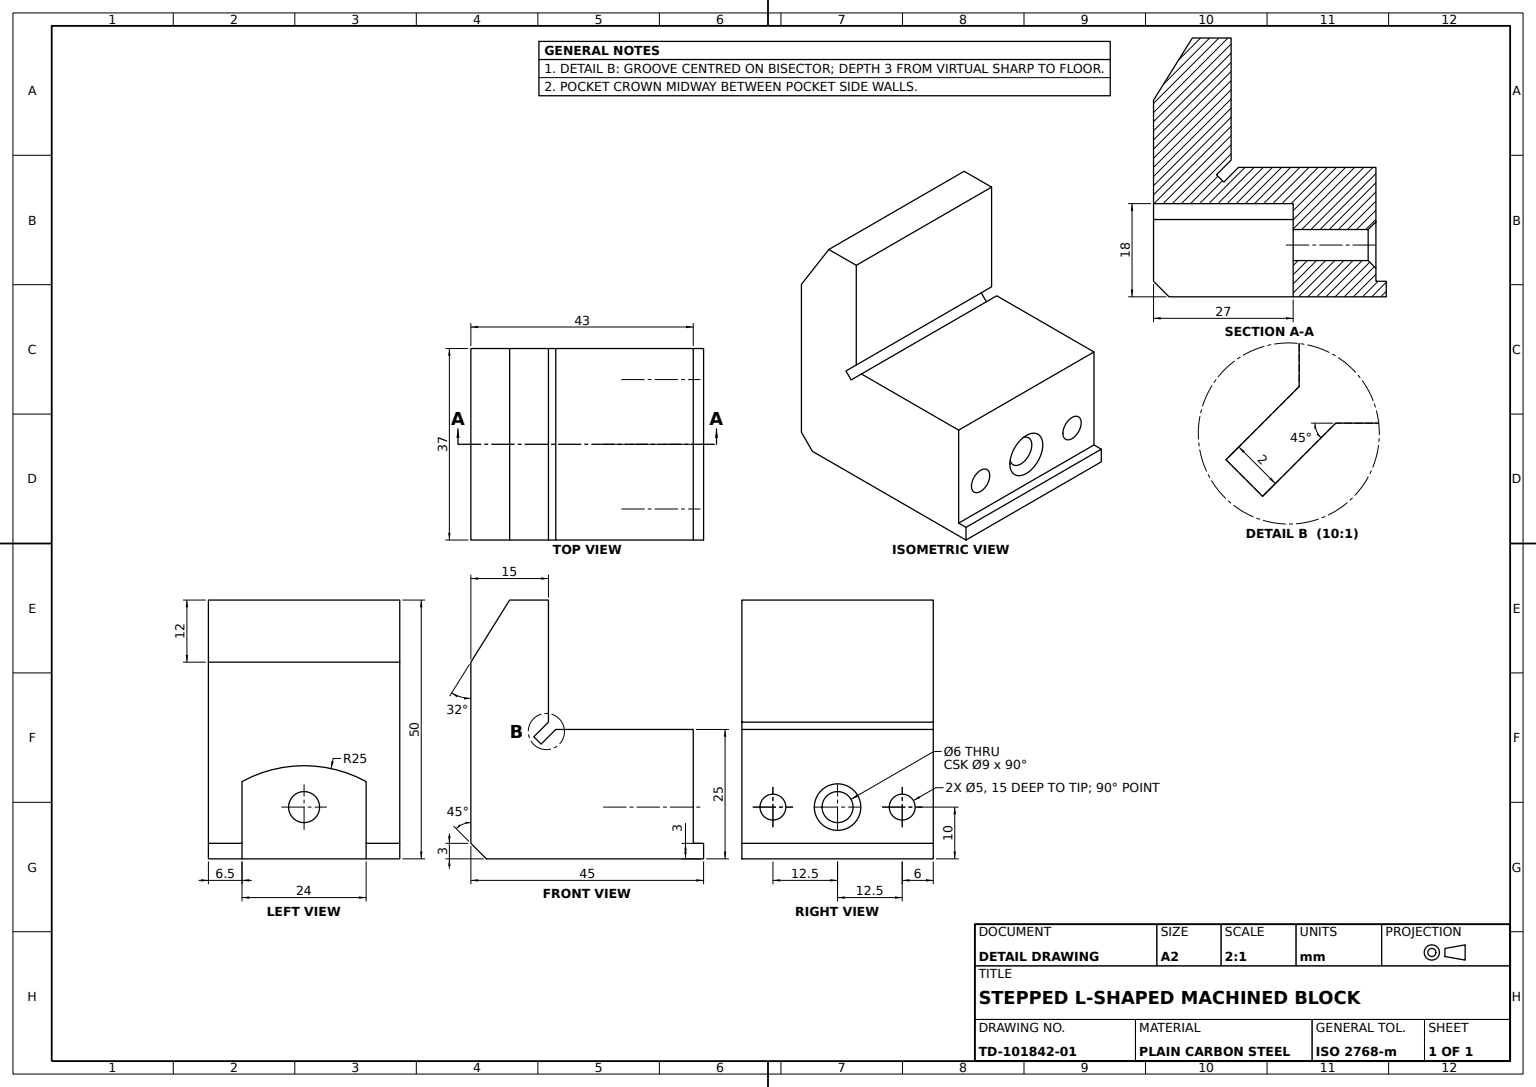
from build123d import *

# Parameters (mm, degrees)
ANCHOR_BLOCK_BODY_DEPTH             = 18.5
TOP_EDGE_CHAMFER_3X45_SIZE          = 3
STEP_GROOVE_DEPTH                   = 64.395583442
STEP_CUT_18_DEEP_DEPTH              = 27
COUNTERSUNK_THRU_HOLE_6_D           = 6
COUNTERSUNK_THRU_HOLE_6_CSINK_D     = 9
COUNTERSUNK_THRU_HOLE_6_CSINK_ANGLE = 90
DRILLED_HOLES_5X15_D                = 5
DRILLED_HOLES_5X15_DEPTH            = 12.5
DRILLED_HOLES_5X15_TIP              = 2.5


with BuildPart() as part:
    # Block Profile Sketch → Anchor Block Body (new, symmetric)
    with BuildSketch(Plane.XY):
        Polygon((0, 0), (0, 13), (7.498432223, 25), (15, 25), (15, 0), (43, 0), (43, -22), (45, -22), (45, -25), (0, -25), align=None)
    extrude(amount=ANCHOR_BLOCK_BODY_DEPTH, both=True)

    # Top Edge Chamfer 3x45
    top_edge_chamfer_3x45_edges = [part.edges().sort_by_distance(p)[0] for p in [
        (0, -25, 0),
    ]]
    chamfer(top_edge_chamfer_3x45_edges, length=TOP_EDGE_CHAMFER_3X45_SIZE)

    # Step Groove Sketch → Step Groove (cut, through all)
    with BuildSketch(Plane.XY.offset(18.5)):
        Polygon((12.878679656, -2.121320344), (12.171572875, -1.414213562), (15, 1.414213562), (16.414213562, 0), (13.585786438, -2.828427125), align=None)
    extrude(amount=-STEP_GROOVE_DEPTH, mode=Mode.SUBTRACT)

    # Step Cut Sketch → Step Cut 18 Deep (cut)
    with BuildSketch(Plane.ZY):
        with BuildLine():
            Line((-12, -25), (-12, -10.068287801))
            ThreePointArc((-12, -10.068287801), (0, -7), (12, -10.068287801))
            Line((12, -10.068287801), (12, -25))
            Line((12, -25), (-12, -25))
        make_face()
    extrude(amount=-STEP_CUT_18_DEEP_DEPTH, mode=Mode.SUBTRACT)

    # Countersunk Thru Hole Ø6 (through all)
    with Locations(Plane(origin=(43, 0, 0), x_dir=(0, 0, -1), z_dir=(1, 0, 0))):
        with Locations((0, -15)):
            CounterSinkHole(COUNTERSUNK_THRU_HOLE_6_D / 2, COUNTERSUNK_THRU_HOLE_6_CSINK_D / 2, counter_sink_angle=COUNTERSUNK_THRU_HOLE_6_CSINK_ANGLE)

    # Drilled Holes Ø5x15
    with Locations(Plane(origin=(43, 0, 0), x_dir=(0, 0, -1), z_dir=(1, 0, 0))):
        with Locations((12.5, -15), (-12.5, -15)):
            Hole(DRILLED_HOLES_5X15_D / 2, depth=DRILLED_HOLES_5X15_DEPTH)
            with Locations((0, 0, -(DRILLED_HOLES_5X15_DEPTH + DRILLED_HOLES_5X15_TIP / 2))):  # 90° drill point
                Cone(0, DRILLED_HOLES_5X15_D / 2, DRILLED_HOLES_5X15_TIP, mode=Mode.SUBTRACT)


solid = part.part
